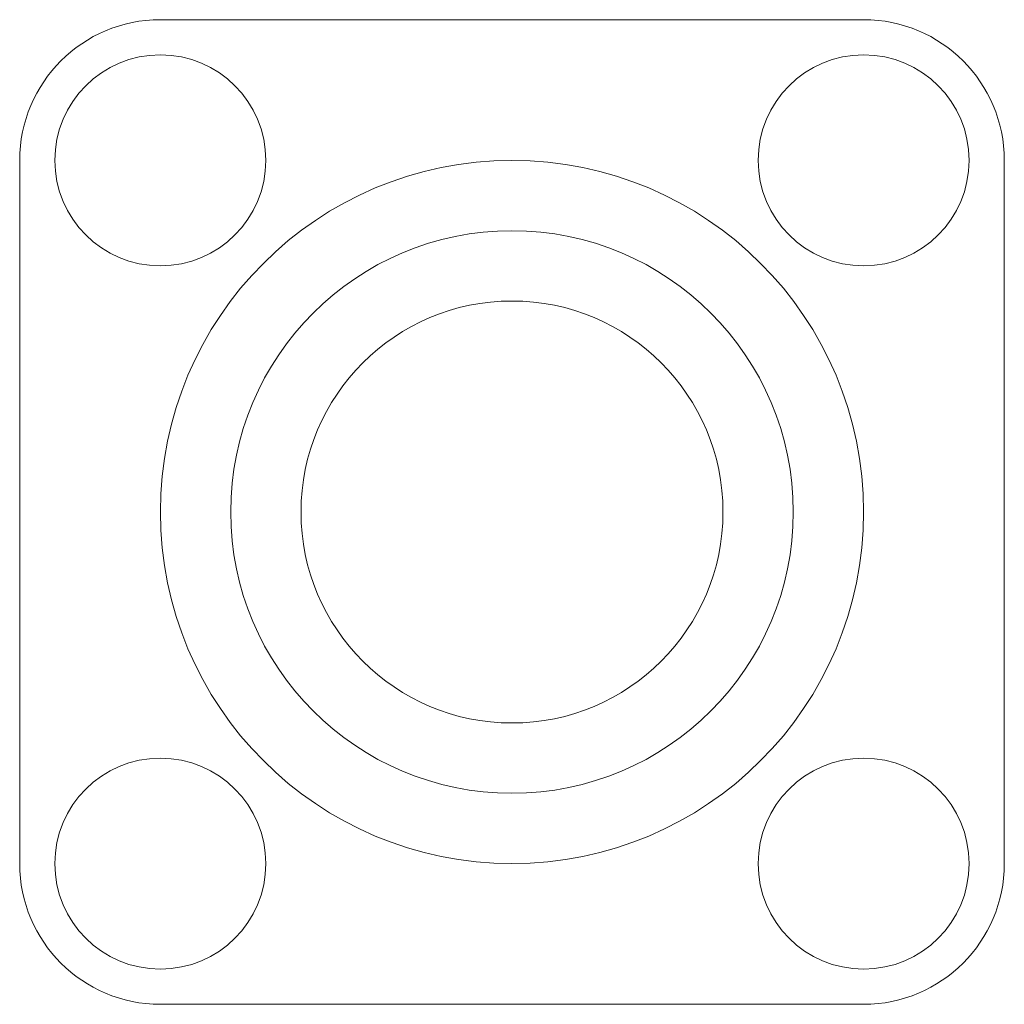
# Model space of a CAD drawing. Units: inches. Extents: x 574.4 to 644.4, y 528 to 598.
import ezdxf

# ---------------------------------------------------------------- set-up
doc = ezdxf.new("R2010")
doc.units = ezdxf.units.IN
doc.header["$MEASUREMENT"] = 0
doc.layers.add('M-CONS', color=8, linetype='Continuous', lineweight=18)

msp = doc.modelspace()

# ---------------------------------------------------------------- linework, layer by layer
at = {"layer": 'M-CONS'}
for points in [[(584.421, 597.956), (634.421, 597.956)], [(574.421, 537.956), (574.421, 587.956)], [(644.421, 587.956), (644.421, 537.956)], [(634.421, 527.956), (584.421, 527.956)]]:
    msp.add_lwpolyline(points, dxfattribs=at)
for centre, radius in [((584.421, 587.956), 7.5), ((634.421, 587.956), 7.5), ((609.421, 562.956, 80), 25), ((609.421, 562.956, 50), 20), ((609.421, 562.956, 10), 15), ((584.421, 537.956), 7.5), ((634.421, 537.956), 7.5)]:
    msp.add_circle(centre, radius, dxfattribs=at)
for centre, start, end in [((584.421, 587.956), 90, 180), ((634.421, 587.956), 0, 90), ((584.421, 537.956), 180, 270), ((634.421, 537.956), 270, 0)]:
    msp.add_arc(centre, 10, start, end, dxfattribs=at)

doc.saveas('drawing.dxf')
